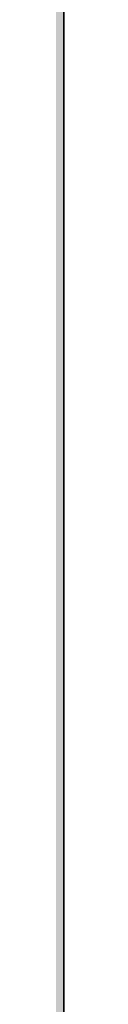
# Model space of a CAD drawing. Units: inches. Extents: x 2083 to 3317, y 1141 to 2115.
# Tile 185 of 256: x 3126.95978 to 3126.95979, y 1263.29018 to 1263.35483. Entities that reach past the tile are written whole.
import ezdxf

# ---------------------------------------------------------------- set-up
doc = ezdxf.new("R2010")
doc.units = ezdxf.units.IN
doc.layers.add('A-ANNO-DIMS', color=2, linetype='Continuous', lineweight=18)
doc.layers.add('A-WALL', color=7, linetype='Continuous', lineweight=35)
doc.layers.add('A-WALL-PATT', color=251, linetype='Continuous', lineweight=13, true_color=0x636466)
doc.styles.get("Standard").update_dxf_attribs({"font": 'arial.ttf'})
doc.dimstyles.new('ISO-25', dxfattribs={"dimtxt": 12, "dimasz": 12, "dimexe": 1.25, "dimexo": 0.625, "dimtad": 1, "dimlunit": 3, "dimtxsty": 'Standard', "dimcen": 2.5, "dimadec": 0, "dimazin": 0, "dimtfac": 1, "dimtmove": 0, "dimatfit": 3, "dimfxl": 1, "dimarcsym": 0})

# ---------------------------------------------------------------- blocks, each defined once
blk = doc.blocks.new('*D9')
at = {"layer": 'A-ANNO-DIMS', "color": 0, "lineweight": -2, "transparency": 16777216}
for p, q in [((3127.584783, 1486.76136), (3190.40309, 1486.76136)), ((3189.15309, 1474.76136), (3189.15309, 1275.26136)), ((3127.584783, 1263.26136), (3190.40309, 1263.26136))]:
    blk.add_line(p, q, dxfattribs=at)
at = {"layer": 'A-ANNO-DIMS', "color": 0, "transparency": 16777216}
for points in [[(3187.15309, 1474.76136), (3191.15309, 1474.76136), (3189.15309, 1486.76136)], [(3187.15309, 1275.26136), (3191.15309, 1275.26136), (3189.15309, 1263.26136)]]:
    blk.add_solid(points, dxfattribs=at)
at = {"layer": 'Defpoints', "color": 0, "transparency": 16777216}
for p in [(3126.959783, 1486.76136), (3126.959783, 1263.26136), (3189.15309, 1263.26136)]:
    blk.add_point(p, dxfattribs=at)
at = {"layer": 'A-ANNO-DIMS', "color": 0, "transparency": 16777216, "insert": (3182.401214, 1375.01136), "char_height": 12, "attachment_point": 5, "rotation": 90}
blk.add_mtext('18\'-7.5"', dxfattribs=at)
blk = doc.blocks.new('*D26')
at = {"layer": 'A-ANNO-DIMS', "color": 0, "lineweight": -2, "transparency": 16777216}
for p, q in [((3088.985844, 1274.915092), (3088.985844, 1270.951963)), ((3111.240037, 1274.915092), (3111.240037, 1270.951963)), ((3076.985844, 1272.201963), (2840.262447, 1272.201963)), ((3111.240037, 1272.201963), (3088.985844, 1272.201963)), ((3123.240037, 1272.201963), (3135.240037, 1272.201963))]:
    blk.add_line(p, q, dxfattribs=at)
at = {"layer": 'A-ANNO-DIMS', "color": 0, "transparency": 16777216}
for points in [[(3076.985844, 1274.201963), (3076.985844, 1270.201963), (3088.985844, 1272.201963)], [(3123.240037, 1274.201963), (3123.240037, 1270.201963), (3111.240037, 1272.201963)]]:
    blk.add_solid(points, dxfattribs=at)
at = {"layer": 'Defpoints', "color": 0, "transparency": 16777216}
for p in [(3088.985844, 1275.540092), (3111.240037, 1275.540092), (3088.985844, 1272.201963)]:
    blk.add_point(p, dxfattribs=at)
at = {"layer": 'A-ANNO-DIMS', "color": 0, "transparency": 16777216, "insert": (2952.624146, 1279.031602), "char_height": 12, "attachment_point": 5}
blk.add_mtext('NIGHTSTAND 1\'-10 1/2" TYP.', dxfattribs=at)
blk = doc.blocks.new('*D27')
at = {"layer": 'A-ANNO-DIMS', "color": 0, "lineweight": -2, "transparency": 16777216}
for p, q in [((3114.578165, 1309.794285), (3114.578165, 1321.794285)), ((3111.865037, 1297.794285), (3115.828165, 1297.794285)), ((3114.578165, 1297.794285), (3114.578165, 1275.540092)), ((3111.865037, 1275.540092), (3115.828165, 1275.540092)), ((3114.578165, 1263.540092), (3114.578165, 1140.988591))]:
    blk.add_line(p, q, dxfattribs=at)
at = {"layer": 'A-ANNO-DIMS', "color": 0, "transparency": 16777216}
for points in [[(3112.578165, 1309.794285), (3116.578165, 1309.794285), (3114.578165, 1297.794285)], [(3112.578165, 1263.540092), (3116.578165, 1263.540092), (3114.578165, 1275.540092)]]:
    blk.add_solid(points, dxfattribs=at)
at = {"layer": 'Defpoints', "color": 0, "transparency": 16777216}
for p in [(3111.240037, 1297.794285), (3111.240037, 1275.540092), (3114.578165, 1275.540092)]:
    blk.add_point(p, dxfattribs=at)
at = {"layer": 'A-ANNO-DIMS', "color": 0, "transparency": 16777216, "insert": (3107.748527, 1196.264342), "char_height": 12, "attachment_point": 5, "rotation": 90}
blk.add_mtext('1\'-10 1/2" TYP.', dxfattribs=at)

msp = doc.modelspace()

# ---------------------------------------------------------------- hatches: boundary and pattern name
at = {"layer": 'A-WALL-PATT'}
h = msp.add_hatch(color=256, dxfattribs=at)
h.dxf.hatch_style = 1
h.paths.add_polyline_path([(3126.959783, 2020.76136), (2748.959783, 2020.76136), (2604.959783, 2020.76136), (2226.959783, 2020.76136), (2226.959783, 1702.76136), (2466.959783, 1702.76136), (2466.959783, 1582.76136), (2418.959783, 1582.76136), (2418.959783, 1477.76136), (2226.959783, 1477.76136), (2226.959783, 1263.26136), (2544.959783, 1263.26136), (2544.959783, 1411.76136), (2604.959783, 1411.76136), (2685.959783, 1411.76136), (2685.959783, 1420.76136), (2604.959783, 1420.76136), (2604.959783, 1573.76136), (2604.959783, 1702.76136), (2604.959783, 2011.76136), (2748.959783, 2011.76136), (2748.959783, 1702.76136), (2862.959783, 1702.76136), (2862.959783, 1621.76136), (2871.959783, 1621.76136), (2871.959783, 1702.76136), (2883.959783, 1702.76136), (2883.959783, 1706.939459, -0.026459), (2883.959783, 1711.76136), (2757.959783, 1711.76136), (2757.959783, 1807.76136), (2787.959783, 1807.76136), (2787.959783, 1812.26136), (2757.959783, 1812.26136), (2757.959783, 2011.76136), (2877.959783, 2011.76136), (2877.959783, 1812.26136), (2847.959783, 1812.26136), (2847.959783, 1807.76136), (2889.835742, 1807.76136), (2889.835742, 1812.26136), (2882.459783, 1812.26136), (2882.459783, 2011.76136), (3117.959783, 2011.76136), (3117.959783, 1812.26136), (2937.835742, 1812.26136), (2937.835742, 1807.76136), (2995.709783, 1807.76136), (2995.709783, 1796.117666), (3000.209783, 1796.117666), (3000.209783, 1807.76136), (3117.959783, 1807.76136), (3117.959783, 1711.76136), (3000.209783, 1711.76136), (3000.209783, 1760.117666), (2998.572705, 1760.117666, -0.020711), (2995.709783, 1760.117666), (2995.709783, 1711.76136), (2931.959783, 1711.76136), (2931.959783, 1702.76136), (3126.959783, 1702.76136)])
h.paths.add_polyline_path([(2471.459783, 2011.76136), (2471.459783, 1810.01136), (2462.716936, 1810.01136), (2462.716936, 1805.51136), (2505.959783, 1805.51136), (2505.959783, 1810.01136), (2475.959783, 1810.01136), (2475.959783, 2011.76136), (2595.959783, 2011.76136), (2595.959783, 1810.01136), (2565.959783, 1810.01136), (2565.959783, 1805.51136), (2595.959783, 1805.51136), (2595.959783, 1711.76136), (2235.959783, 1711.76136), (2235.959783, 1805.51136), (2353.709783, 1805.51136), (2353.709783, 1796.054162), (2358.209783, 1796.054162), (2358.209783, 1805.51136), (2414.716936, 1805.51136), (2414.716936, 1810.01136), (2235.959783, 1810.01136), (2235.959783, 2011.76136)], flags=16)
h.paths.add_polyline_path([(2270.204734, 1994.610008), (2270.204734, 1970.610008), (2246.204734, 1970.610008), (2246.204734, 1994.610008)], flags=0)
edge = h.paths.add_edge_path(flags=0)
edge.add_ellipse((2332.027391, 1899.798176), major_axis=(-3.042994, 3.042994), ratio=0.16825245, start_angle=-161.332166, end_angle=-156.307114, ccw=False)
edge.add_ellipse((2333.082037, 1898.74353), major_axis=(-1.054646, 1.054646), ratio=0.4535321, start_angle=-123.371019, end_angle=-94.159107)
edge = h.paths.add_edge_path(flags=0)
edge.add_ellipse((2332.027391, 1968.87629), major_axis=(3.042994, 3.042994), ratio=0.16825245, start_angle=18.667834, end_angle=23.692886)
edge.add_spline(control_points=[(2332.925596, 1970.691105), (2332.226768, 1970.3361), (2330.893709, 1969.658905), (2328.41308, 1970.932138), (2327.203934, 1967.748712), (2324.709596, 1969.955589), (2322.532822, 1967.012354), (2320.012846, 1971.295812), (2317.680308, 1968.157845), (2316.040526, 1967.102047), (2315.426904, 1966.809602)], knot_values=[0, 0, 0, 0, 2.267059, 4.324559, 6.685584, 8.878641, 11.121502, 14.300359, 17.755284, 19.732645, 19.732645, 19.732645, 19.732645], degree=3, periodic=0)
edge.add_ellipse((2332.027391, 1968.87629), major_axis=(3.042994, 3.042994), ratio=0.16825245, start_angle=18.667834, end_angle=23.692886, ccw=False)
edge.add_ellipse((2333.082037, 1969.930936), major_axis=(1.054646, 1.054646), ratio=0.4535321, start_angle=56.628981, end_angle=85.840893, ccw=False)
edge = h.paths.add_edge_path(flags=0)
edge.add_spline(control_points=[(2296.428287, 1967.987908), (2293.627804, 1965.336314), (2287.703624, 1959.727094), (2299.74386, 1949.995699), (2294.532591, 1935.668528), (2290.573228, 1920.603512), (2293.394124, 1909.973691), (2296.185407, 1904.966543)], knot_values=[0.099185, 0.099185, 0.099185, 0.099185, 0.345301, 0.619822, 0.982653, 1.386093, 1.810555, 1.810555, 1.810555, 1.810555], degree=3, periodic=0)
edge.add_spline(control_points=[(2296.185407, 1904.966543), (2297.383582, 1902.6193), (2298.000969, 1901.949312), (2298.55297, 1901.468155)], knot_values=[0.006246, 0.006246, 0.006246, 0.006246, 0.055476, 0.055476, 0.055476, 0.055476], degree=3, periodic=0)
edge.add_spline(control_points=[(2298.55297, 1901.468155), (2297.258612, 1900.923224), (2295.225294, 1900.232126), (2293.060229, 1900.614205), (2292.101423, 1900.788415), (2292.089578, 1900.790568)], knot_values=[0.312835, 0.312835, 0.312835, 0.312835, 0.40178, 0.474987, 0.475903, 0.475903, 0.475903, 0.475903], degree=3, periodic=0)
edge.add_arc((2292.793646, 1904.664109), 3.937008, 215.420897, 259.698179, ccw=False)
edge.add_spline(control_points=[(2289.585314, 1902.382304), (2289.476652, 1902.535087), (2289.36848, 1902.688035), (2289.260865, 1902.84117)], knot_values=[0.102872, 0.102872, 0.102872, 0.102872, 0.116896, 0.116896, 0.116896, 0.116896], degree=3, periodic=0)
edge.add_spline(control_points=[(2289.260865, 1902.84117), (2288.686604, 1902.550192), (2287.640048, 1902.019902), (2285.881337, 1901.873954), (2283.852972, 1901.504352), (2281.719987, 1899.710538), (2278.466991, 1899.492942), (2276.157136, 1901.883202), (2272.258953, 1899.804071), (2267.777605, 1901.843183), (2262.243882, 1900.184033), (2257.414927, 1901.782061), (2254.318374, 1900.72612), (2253.178285, 1900.337343)], knot_values=[0, 0, 0, 0, 1.907977, 3.477176, 5.261074, 7.972851, 11.680248, 13.717921, 16.939592, 22.789562, 27.502503, 33.595215, 37.145618, 37.145618, 37.145618, 37.145618], degree=3, periodic=0)
edge.add_line((2253.178285, 1900.337343), (2250.24424, 1902.84117))
edge.add_line((2250.24424, 1902.84117), (2250.24424, 1965.833296))
edge.add_line((2250.24424, 1965.833296), (2253.178285, 1968.337123))
edge.add_spline(control_points=[(2253.178285, 1968.337123), (2254.318374, 1967.948346), (2257.414927, 1966.892405), (2262.243882, 1968.490433), (2267.777605, 1966.831283), (2271.52673, 1968.537217), (2273.875914, 1967.828289), (2274.206701, 1967.727642)], knot_values=[0, 0, 0, 0, 0.09018, 0.244935, 0.364644, 0.513233, 0.537855, 0.537855, 0.537855, 0.537855], degree=3, periodic=0)
edge.add_arc((2274.352887, 1963.793349), 3.937008, 72.051134, 92.127949, ccw=False)
edge.add_arc((2281.296933, 1985.230003), 18.596298, 252.0511336, 288.5657217)
edge.add_arc((2292.316717, 1956.02888), 12.646081, 71.0267879, 113.7782184, ccw=False)
edge = h.paths.add_edge_path(flags=0)
edge.add_spline(control_points=[(2274.899415, 1951.856195), (2275.066156, 1951.616592), (2275.232687, 1951.376588), (2275.397987, 1951.135855)], knot_values=[1.409916, 1.409916, 1.409916, 1.409916, 1.43159, 1.43159, 1.43159, 1.43159], degree=3, periodic=0)
edge.add_spline(control_points=[(2275.397987, 1951.135855), (2275.792106, 1950.561885), (2276.179231, 1949.983774), (2276.545546, 1949.397103)], knot_values=[1.358238, 1.358238, 1.358238, 1.358238, 1.409916, 1.409916, 1.409916, 1.409916], degree=3, periodic=0)
edge.add_line((2276.545546, 1949.397103), (2277.437289, 1947.862185))
edge.add_spline(control_points=[(2277.437289, 1947.862185), (2276.303834, 1945.673115), (2274.639698, 1942.426882), (2274.631615, 1938.0939), (2272.799124, 1930.85155), (2274.356426, 1943.897046), (2275.947681, 1947.923356), (2276.545546, 1949.397103)], knot_values=[0.005632, 0.005632, 0.005632, 0.005632, 0.186014, 0.266002, 0.357087, 0.59639, 0.739732, 0.739732, 0.739732, 0.739732], degree=3, periodic=0)
edge.add_spline(control_points=[(2276.545546, 1949.397103), (2276.179231, 1949.983774), (2275.792106, 1950.561885), (2275.397987, 1951.135855)], knot_values=[1.358238, 1.358238, 1.358238, 1.358238, 1.409916, 1.409916, 1.409916, 1.409916], degree=3, periodic=0)
edge.add_spline(control_points=[(2275.397987, 1951.135855), (2274.9425, 1950.080452), (2274.20776, 1948.025272), (2273.934602, 1944.851477), (2272.468534, 1937.627489), (2273.466216, 1945.696466), (2274.700615, 1951.059472), (2274.899415, 1951.856195)], knot_values=[0.104364, 0.104364, 0.104364, 0.104364, 0.189636, 0.269624, 0.36071, 0.600013, 0.644622, 0.644622, 0.644622, 0.644622], degree=3, periodic=0)
h.paths.add_polyline_path([(2269.167514, 1963.127573, -0.357527), (2268.170633, 1960.97637, -0.092561), (2268.170633, 1939.436325, -0.357527), (2269.167514, 1937.285122, -0.357527), (2267.01631, 1938.282002, -0.164785), (2254.685581, 1938.282002, -0.357527), (2252.534378, 1937.285122, -0.357527), (2253.531259, 1939.436325, -0.092561), (2253.531259, 1960.97637, -0.357527), (2252.534378, 1963.127573, -0.357527), (2254.685581, 1962.130692, -0.164785), (2267.01631, 1962.130692, -0.357527)], flags=0)
h.paths.add_polyline_path([(2248.874068, 1967.8018), (2248.874068, 1957.02771), (2249.457783, 1957.02771), (2249.457783, 1911.646756), (2248.874068, 1911.646756), (2248.874068, 1900.872666), (2246.511863, 1900.872666, 0.197327), (2244.149658, 1902.456873), (2244.149658, 1966.217592, 0.197327), (2246.511863, 1967.8018)], flags=0)
h.paths.add_polyline_path([(2269.167514, 1931.389344, -0.357527), (2268.170633, 1929.238141, -0.092561), (2268.170633, 1907.698096, -0.357527), (2269.167514, 1905.546893, -0.357527), (2267.01631, 1906.543774, -0.164785), (2254.685581, 1906.543774, -0.357527), (2252.534378, 1905.546893, -0.357527), (2253.531259, 1907.698096, -0.092561), (2253.531259, 1929.238141, -0.357527), (2252.534378, 1931.389344, -0.357527), (2254.685581, 1930.392463, -0.164785), (2267.01631, 1930.392463, -0.357527)], flags=0)
edge = h.paths.add_edge_path(flags=0)
edge.add_spline(control_points=[(2276.196858, 1906.723702), (2276.168144, 1909.028928), (2276.114049, 1913.371852), (2270.598417, 1924.924978), (2273.905175, 1919.012779), (2275.921711, 1916.262063), (2275.47457, 1912.402149), (2277.257874, 1910.380621), (2276.696044, 1908.225036), (2276.646218, 1906.813023), (2276.617825, 1906.008407)], knot_values=[0, 0, 0, 0, 8.61026, 16.221274, 18.843057, 23.804898, 27.440828, 29.356102, 31.203478, 33.650687, 33.650687, 33.650687, 33.650687], degree=3, periodic=0)
edge.add_spline(control_points=[(2276.617825, 1906.008407), (2276.623313, 1905.624144), (2276.497738, 1904.628661), (2275.441779, 1903.854725), (2274.937314, 1903.08045), (2274.85908, 1902.84117)], knot_values=[0.156488, 0.156488, 0.156488, 0.156488, 0.184398, 0.231376, 0.250598, 0.250598, 0.250598, 0.250598], degree=3, periodic=0)
edge.add_line((2274.85908, 1902.84117), (2276.50598, 1902.84117))
edge.add_spline(control_points=[(2276.50598, 1902.84117), (2276.788308, 1903.08494), (2277.665071, 1904.125196), (2278.249538, 1904.340738), (2277.653872, 1908.527387), (2278.15567, 1906.227808), (2278.100464, 1905.285948), (2278.846675, 1904.069005), (2277.856785, 1903.414948), (2277.874191, 1902.99105), (2277.903562, 1902.84117)], knot_values=[0.059574, 0.059574, 0.059574, 0.059574, 0.080753, 0.103741, 0.16972, 0.176036, 0.207137, 0.240474, 0.262341, 0.27366, 0.27366, 0.27366, 0.27366], degree=3, periodic=0)
edge.add_line((2277.903562, 1902.84117), (2280.029825, 1902.84117))
edge.add_spline(control_points=[(2280.029825, 1902.84117), (2279.888221, 1903.088398), (2279.499257, 1903.981551), (2280.152284, 1905.939349), (2278.103615, 1909.657757), (2279.762395, 1907.185285), (2280.3279, 1904.874861), (2280.485109, 1903.48959), (2281.463269, 1903.249432), (2281.758343, 1902.936497), (2281.834036, 1902.84117)], knot_values=[0.013856, 0.013856, 0.013856, 0.013856, 0.034874, 0.088867, 0.107879, 0.126738, 0.158714, 0.193757, 0.217487, 0.226722, 0.226722, 0.226722, 0.226722], degree=3, periodic=0)
edge.add_spline(control_points=[(2281.834036, 1902.84117), (2281.787535, 1902.826703), (2281.647022, 1902.782988), (2281.395527, 1902.85949), (2281.088077, 1902.985242), (2280.720683, 1903.060902), (2280.333451, 1903.025726), (2280.124767, 1902.898879), (2280.029825, 1902.84117)], knot_values=[0, 0, 0, 0, 0.14413, 0.435517, 0.749276, 1.153046, 1.548371, 1.878348, 1.878348, 1.878348, 1.878348], degree=3, periodic=0)
edge.add_line((2280.029825, 1902.84117), (2277.903562, 1902.84117))
edge.add_spline(control_points=[(2277.903562, 1902.84117), (2277.892855, 1902.795855), (2277.865396, 1902.679637), (2277.607479, 1902.687483), (2277.27405, 1902.8007), (2276.837921, 1902.619775), (2276.583807, 1902.789261), (2276.50598, 1902.84117)], knot_values=[0, 0, 0, 0, 0.127189, 0.326199, 0.628009, 1.24357, 1.515331, 1.515331, 1.515331, 1.515331], degree=3, periodic=0)
edge.add_line((2276.50598, 1902.84117), (2274.85908, 1902.84117))
edge.add_spline(control_points=[(2274.85908, 1902.84117), (2274.814437, 1902.898587), (2274.72513, 1903.013446), (2274.493477, 1903.118968), (2274.244285, 1902.960539), (2273.937121, 1903.184942), (2273.614039, 1902.983143), (2273.408316, 1902.883045), (2273.322254, 1902.84117)], knot_values=[0, 0, 0, 0, 0.21843, 0.436957, 0.687977, 0.990379, 1.398396, 1.69185, 1.69185, 1.69185, 1.69185], degree=3, periodic=0)
edge.add_spline(control_points=[(2273.322254, 1902.84117), (2273.61674, 1903.445692), (2274.273998, 1904.538253), (2276.027239, 1904.573702), (2276.206963, 1906.583637), (2276.196858, 1906.723702)], knot_values=[0.012227, 0.012227, 0.012227, 0.012227, 0.059472, 0.106218, 0.134458, 0.134458, 0.134458, 0.134458], degree=3, periodic=0)
h.paths.add_polyline_path([(2270.776054, 1897.789828), (2270.776054, 1873.789828), (2246.776054, 1873.789828), (2246.776054, 1897.789828)], flags=0)
h.paths.add_polyline_path([(2353.709783, 1760.005059), (2353.709783, 1760.054162), (2358.209783, 1760.054162, -0.033729)], flags=0)
h.paths.add_polyline_path([(2321.819119, 1737.529186), (2341.995327, 1737.529186, -0.414214), (2343.203273, 1736.321241), (2343.203273, 1721.020596, -0.414214), (2341.995327, 1719.812651), (2321.819119, 1719.812651, -0.414214), (2320.611173, 1721.020596), (2320.611173, 1736.321241, -0.414214)], flags=0)
h.paths.add_polyline_path([(2324.23501, 1736.321241), (2339.579436, 1736.321241, -0.414214), (2341.995327, 1733.905349), (2341.995327, 1725.44973, -0.414214), (2339.579436, 1723.033839), (2333.680588, 1723.033839), (2333.845317, 1722.045467, -0.870646), (2335.425399, 1721.825893, -0.767327), (2333.922694, 1721.423245), (2331.291024, 1721.423245, -0.767327), (2329.788319, 1721.825893, -0.870646), (2331.368401, 1722.045467), (2331.53313, 1723.033839), (2324.23501, 1723.033839, -0.414214), (2321.819119, 1725.44973), (2321.819119, 1733.905349, -0.414214)], flags=0)
h.paths.add_polyline_path([(2570.483789, 1928.615444), (2589.683789, 1928.615444), (2590.168829, 1928.615444), (2590.168829, 1904.993397), (2570.483789, 1904.993397)], flags=0)
h.paths.add_polyline_path([(2574.447324, 1927.263822, -1), (2572.828836, 1927.263822, -1)], flags=0)
h.paths.add_polyline_path([(2573.089867, 1926.940877), (2573.925032, 1927.776042), (2574.147743, 1927.553332), (2573.312577, 1926.718166)], flags=0)
h.paths.add_polyline_path([(2578.779065, 1919.729618, -1), (2571.591663, 1919.729618, -1)], flags=0)
h.paths.add_polyline_path([(2578.385364, 1919.729618, -1), (2571.985364, 1919.729618, -1)], flags=0)
h.paths.add_polyline_path([(2331.595764, 1729.476216, -1), (2333.617954, 1729.476216, -1)], flags=0)
h.paths.add_polyline_path([(2578.034228, 1927.263822, -1), (2576.41574, 1927.263822, -1)], flags=0)
h.paths.add_polyline_path([(2576.688851, 1927.531089), (2576.911562, 1927.753799), (2577.746728, 1926.918634), (2577.524017, 1926.695923)], flags=0)
h.paths.add_polyline_path([(2578.139065, 1909.859539, -1), (2572.231663, 1909.859539, -1)], flags=0)
h.paths.add_polyline_path([(2577.745364, 1909.859539, -1), (2572.625364, 1909.859539, -1)], flags=0)
h.paths.add_polyline_path([(2583.797718, 1927.263822, -1), (2582.179229, 1927.263822, -1)], flags=0)
h.paths.add_polyline_path([(2582.718649, 1927.753799), (2583.553814, 1926.918634), (2583.331103, 1926.695923), (2582.495938, 1927.531089)], flags=0)
h.paths.add_polyline_path([(2582.495938, 1927.531089), (2582.718649, 1927.753799), (2583.553814, 1926.918634), (2583.331103, 1926.695923)], flags=0)
h.paths.add_polyline_path([(2587.739065, 1920.529618, -1), (2581.831663, 1920.529618, -1)], flags=0)
h.paths.add_polyline_path([(2587.345364, 1920.529618, -1), (2582.225364, 1920.529618, -1)], flags=0)
h.paths.add_polyline_path([(2587.384622, 1927.263822, -1), (2585.766133, 1927.263822, -1)], flags=0)
h.paths.add_polyline_path([(2586.081993, 1926.980247), (2586.917158, 1927.815412), (2587.139869, 1927.592702), (2586.304703, 1926.757536)], flags=0)
h.paths.add_polyline_path([(2588.379065, 1910.659539, -1), (2581.191663, 1910.659539, -1)], flags=0)
h.paths.add_polyline_path([(2587.985364, 1910.659539, -1), (2581.585364, 1910.659539, -1)], flags=0)
h.paths.add_polyline_path([(2417.167729, 1729.477895), (2437.343937, 1729.477895, -0.414214), (2438.551883, 1728.26995), (2438.551883, 1712.969306, -0.414214), (2437.343937, 1711.76136), (2417.167729, 1711.76136, -0.414214), (2415.959783, 1712.969306), (2415.959783, 1728.26995, -0.414214)], flags=0)
h.paths.add_polyline_path([(2419.58362, 1728.26995), (2434.928046, 1728.26995, -0.414214), (2437.343937, 1725.854059), (2437.343937, 1717.39844, -0.414214), (2434.928046, 1714.982548), (2429.029199, 1714.982548), (2429.193927, 1713.994176, -0.870646), (2430.774009, 1713.774603, -0.767327), (2429.271304, 1713.371954), (2426.639634, 1713.371954, -0.767327), (2425.136929, 1713.774603, -0.870646), (2426.717011, 1713.994176), (2426.88174, 1714.982548), (2419.58362, 1714.982548, -0.414214), (2417.167729, 1717.39844), (2417.167729, 1725.854059, -0.414214)], flags=0)
h.paths.add_polyline_path([(2419.58362, 1728.26995), (2434.928046, 1728.26995, -0.414214), (2437.343937, 1725.854059), (2437.343937, 1717.39844, -0.414214), (2434.928046, 1714.982548), (2429.029199, 1714.982548), (2428.358118, 1719.009034), (2427.552821, 1719.009034), (2426.88174, 1714.982548), (2419.58362, 1714.982548, -0.414214), (2417.167729, 1717.39844), (2417.167729, 1725.854059, -0.414214)], flags=0)
h.paths.add_polyline_path([(2426.944374, 1721.424925, -1), (2428.966564, 1721.424925, -1)], flags=0)
h.paths.add_polyline_path([(2475.959783, 1702.76136), (2595.959783, 1702.76136), (2595.959783, 1582.76136), (2475.959783, 1582.76136)], flags=16)
h.paths.add_polyline_path([(2427.959783, 1573.76136), (2595.959783, 1573.76136), (2595.959783, 1468.76136), (2595.959783, 1420.76136), (2384.459783, 1420.76136), (2384.459783, 1468.76136), (2427.959783, 1468.76136)], flags=16)
h.paths.add_polyline_path([(2379.959783, 1468.76136), (2379.959783, 1420.76136), (2235.959783, 1420.76136), (2235.959783, 1468.76136)], flags=16)
h.paths.add_polyline_path([(2317.815996, 1466.695767), (2337.992205, 1466.695767, -0.414214), (2339.20015, 1465.487821), (2339.20015, 1450.187177, -0.414214), (2337.992205, 1448.979232), (2317.815996, 1448.979232, -0.414214), (2316.608051, 1450.187177), (2316.608051, 1465.487821, -0.414214)], flags=0)
h.paths.add_polyline_path([(2320.231887, 1465.487821), (2335.576313, 1465.487821, -0.414214), (2337.992205, 1463.07193), (2337.992205, 1454.616311, -0.414214), (2335.576313, 1452.20042), (2329.677466, 1452.20042), (2329.842195, 1451.212047, -0.870646), (2331.422276, 1450.992474, -0.767327), (2329.919571, 1450.589826), (2327.287902, 1450.589826, -0.767327), (2325.785197, 1450.992474, -0.870646), (2327.365278, 1451.212047), (2327.530007, 1452.20042), (2320.231887, 1452.20042, -0.414214), (2317.815996, 1454.616311), (2317.815996, 1463.07193, -0.414214)], flags=0)
h.paths.add_polyline_path([(2320.231887, 1465.487821), (2335.576313, 1465.487821, -0.414214), (2337.992205, 1463.07193), (2337.992205, 1454.616311, -0.414214), (2335.576313, 1452.20042), (2329.677466, 1452.20042), (2329.006385, 1456.226905), (2328.201088, 1456.226905), (2327.530007, 1452.20042), (2320.231887, 1452.20042, -0.414214), (2317.815996, 1454.616311), (2317.815996, 1463.07193, -0.414214)], flags=0)
h.paths.add_polyline_path([(2327.592641, 1458.642796, -1), (2329.614832, 1458.642796, -1)], flags=0)
h.paths.add_polyline_path([(2244.411744, 1433.340453), (2241.920945, 1433.340453, -0.414214), (2240.017856, 1435.243542), (2240.017856, 1440.952808, -0.414211), (2241.920925, 1442.855897), (2244.411744, 1442.855897, -1.976472)], flags=0)
h.paths.add_polyline_path([(2245.356888, 1434.397536, -0.414214), (2245.356888, 1441.798814, -2.144098)], flags=0)
h.paths.add_polyline_path([(2535.959783, 1416.26136), (2535.959783, 1272.26136), (2235.959783, 1272.26136), (2235.959783, 1416.26136)], flags=16)
h.paths.add_polyline_path([(2260.119561, 1384.292841), (2260.119561, 1362.038649), (2237.865369, 1362.038649), (2237.865369, 1384.292841)], flags=0)
edge = h.paths.add_edge_path(flags=0)
edge.add_line((2318.251847, 1362.093298), (2318.145797, 1362.000973))
edge.add_ellipse((2317.445116, 1360.431044), major_axis=(2.82164, 2.82164), ratio=0.16825245, start_angle=18.667834, end_angle=20.948127, ccw=False)
edge.add_ellipse((2318.423045, 1361.408974), major_axis=(0.977929, 0.977929), ratio=0.4535321, start_angle=56.628981, end_angle=70.226201, ccw=False)
edge = h.paths.add_edge_path(flags=0)
edge.add_line((2319.10737, 1295.571078), (2319.015044, 1295.677128))
edge.add_ellipse((2317.445116, 1296.377809), major_axis=(-2.82164, 2.82164), ratio=0.16825245, start_angle=-161.332166, end_angle=-159.051873, ccw=False)
edge.add_ellipse((2318.423045, 1295.39988), major_axis=(-0.977929, 0.977929), ratio=0.4535321, start_angle=-123.371019, end_angle=-109.773799)
edge = h.paths.add_edge_path(flags=0)
edge.add_spline(control_points=[(2284.210349, 1301.170219), (2284.580688, 1300.444719), (2284.891189, 1299.892024), (2285.159553, 1299.461018)], knot_values=[0.039066, 0.039066, 0.039066, 0.039066, 0.055476, 0.055476, 0.055476, 0.055476], degree=3, periodic=0)
edge.add_line((2285.159553, 1299.461018), (2284.210349, 1301.170219))
edge = h.paths.add_edge_path(flags=0)
edge.add_line((2280.412458, 1297.298013), (2283.369991, 1297.036122))
edge.add_line((2283.369991, 1297.036122), (2286.40569, 1297.92631))
edge.add_spline(control_points=[(2286.40569, 1297.92631), (2285.305487, 1297.463119), (2284.344777, 1297.129151), (2283.369991, 1297.036122)], knot_values=[0.394369, 0.394369, 0.394369, 0.394369, 0.475903, 0.475903, 0.475903, 0.475903], degree=3, periodic=0)
edge.add_spline(control_points=[(2283.369991, 1297.036122), (2283.28139, 1297.027666), (2282.316289, 1296.957336), (2281.312502, 1297.134479), (2280.423441, 1297.296016), (2280.412458, 1297.298013)], knot_values=[0.312835, 0.312835, 0.312835, 0.312835, 0.320246, 0.393453, 0.394369, 0.394369, 0.394369, 0.394369], degree=3, periodic=0)
edge = h.paths.add_edge_path(flags=0)
edge.add_line((2284.435561, 1359.607285), (2280.446291, 1355.328047))
edge.add_line((2280.446291, 1355.328047), (2279.579987, 1351.017754))
edge.add_line((2279.579987, 1351.017754), (2282.412974, 1346.580433))
edge.add_spline(control_points=[(2282.412974, 1346.580433), (2283.153331, 1345.589236), (2284.252896, 1344.028897), (2284.801037, 1342.387167), (2284.935162, 1341.805544)], knot_values=[1.240098, 1.240098, 1.240098, 1.240098, 1.332892, 1.382712, 1.382712, 1.382712, 1.382712], degree=3, periodic=0)
edge.add_spline(control_points=[(2284.935162, 1341.805544), (2285.319108, 1340.1406), (2285.233029, 1338.409204), (2284.909938, 1336.654122)], knot_values=[1.097484, 1.097484, 1.097484, 1.097484, 1.240098, 1.240098, 1.240098, 1.240098], degree=3, periodic=0)
edge.add_spline(control_points=[(2284.909938, 1336.654122), (2284.586848, 1334.89904), (2284.026745, 1333.120272), (2283.462644, 1331.360585)], knot_values=[0.95487, 0.95487, 0.95487, 0.95487, 1.097484, 1.097484, 1.097484, 1.097484], degree=3, periodic=0)
edge.add_line((2283.462644, 1331.360585), (2281.890376, 1326.153357))
edge.add_line((2281.890376, 1326.153357), (2280.756259, 1321.056089))
edge.add_line((2280.756259, 1321.056089), (2280.299205, 1316.001977))
edge.add_line((2280.299205, 1316.001977), (2280.715933, 1310.950068))
edge.add_line((2280.715933, 1310.950068), (2282.028094, 1305.972137))
edge.add_line((2282.028094, 1305.972137), (2284.210349, 1301.170219))
edge.add_spline(control_points=[(2284.210349, 1301.170219), (2283.340731, 1302.730185), (2282.611904, 1304.336493), (2282.028094, 1305.972137)], knot_values=[0.099185, 0.099185, 0.099185, 0.099185, 0.241799, 0.241799, 0.241799, 0.241799], degree=3, periodic=0)
edge.add_spline(control_points=[(2282.028094, 1305.972137), (2281.444283, 1307.60778), (2281.005489, 1309.272759), (2280.715933, 1310.950068)], knot_values=[0.241799, 0.241799, 0.241799, 0.241799, 0.384413, 0.384413, 0.384413, 0.384413], degree=3, periodic=0)
edge.add_spline(control_points=[(2280.715933, 1310.950068), (2280.433241, 1312.587613), (2280.289386, 1314.276959), (2280.298894, 1315.962032), (2280.299205, 1316.001977)], knot_values=[0.384413, 0.384413, 0.384413, 0.384413, 0.523647, 0.527028, 0.527028, 0.527028, 0.527028], degree=3, periodic=0)
edge.add_spline(control_points=[(2280.299205, 1316.001977), (2280.312326, 1317.686955), (2280.477871, 1319.367926), (2280.756259, 1321.056089)], knot_values=[0.527028, 0.527028, 0.527028, 0.527028, 0.669642, 0.669642, 0.669642, 0.669642], degree=3, periodic=0)
edge.add_spline(control_points=[(2280.756259, 1321.056089), (2281.034648, 1322.744252), (2281.42588, 1324.439608), (2281.890376, 1326.153357)], knot_values=[0.669642, 0.669642, 0.669642, 0.669642, 0.812256, 0.812256, 0.812256, 0.812256], degree=3, periodic=0)
edge.add_spline(control_points=[(2281.890376, 1326.153357), (2282.264383, 1327.533251), (2282.78787, 1329.26181), (2283.352751, 1331.01778), (2283.462644, 1331.360585)], knot_values=[0.812256, 0.812256, 0.812256, 0.812256, 0.927087, 0.95487, 0.95487, 0.95487, 0.95487], degree=3, periodic=0)
edge.add_line((2283.462644, 1331.360585), (2284.909938, 1336.654122))
edge.add_line((2284.909938, 1336.654122), (2284.935162, 1341.805544))
edge.add_line((2284.935162, 1341.805544), (2282.412974, 1346.580433))
edge.add_spline(control_points=[(2282.412974, 1346.580433), (2281.275127, 1348.103792), (2280.078447, 1349.570318), (2279.579987, 1351.017754)], knot_values=[1.382712, 1.382712, 1.382712, 1.382712, 1.525326, 1.525326, 1.525326, 1.525326], degree=3, periodic=0)
edge.add_spline(control_points=[(2279.579987, 1351.017754), (2279.443282, 1351.414721), (2279.136312, 1352.856922), (2279.73519, 1354.290385), (2280.446291, 1355.328047)], knot_values=[1.525326, 1.525326, 1.525326, 1.525326, 1.564439, 1.667941, 1.667941, 1.667941, 1.667941], degree=3, periodic=0)
edge.add_spline(control_points=[(2280.446291, 1355.328047), (2281.426113, 1356.757835), (2282.930837, 1358.18256), (2284.435561, 1359.607285)], knot_values=[1.667941, 1.667941, 1.667941, 1.667941, 1.810555, 1.810555, 1.810555, 1.810555], degree=3, periodic=0)
edge.add_arc((2280.623075, 1348.518181), 11.72618, 71.0267879, 113.7782184)
edge.add_arc((2270.404892, 1375.595156), 17.243567, 252.0511336, 288.5657217, ccw=False)
edge.add_arc((2263.965969, 1355.717847), 3.650622, 72.051134, 92.127949)
edge.add_arc((2263.965969, 1355.717847), 3.650622, 92.127949, 177.98513)
edge.add_spline(control_points=[(2260.317604, 1355.846199), (2260.260417, 1354.220668), (2260.551278, 1350.186547), (2262.999344, 1346.766251), (2264.472741, 1344.649024)], knot_values=[1.43159, 1.43159, 1.43159, 1.43159, 1.564144, 1.770695, 1.770695, 1.770695, 1.770695], degree=3, periodic=0)
edge.add_line((2264.472741, 1344.649024), (2264.93559, 1343.98253))
edge.add_spline(control_points=[(2263.801044, 1340.248105), (2263.843238, 1340.514088), (2264.067244, 1341.756465), (2264.512693, 1343.002453), (2264.935047, 1343.981083)], knot_values=[0.53657, 0.53657, 0.53657, 0.53657, 0.559349, 0.644622, 0.644622, 0.644622, 0.644622], degree=3, periodic=0)
edge.add_spline(control_points=[(2264.935047, 1343.981083), (2265.117771, 1343.714975), (2265.298875, 1343.447906), (2265.476756, 1343.179365)], knot_values=[1.384077, 1.384077, 1.384077, 1.384077, 1.409916, 1.409916, 1.409916, 1.409916], degree=3, periodic=0)
edge.add_spline(control_points=[(2265.476756, 1343.179365), (2265.654637, 1342.910823), (2265.829296, 1342.64081), (2265.99913, 1342.368812)], knot_values=[1.358238, 1.358238, 1.358238, 1.358238, 1.384077, 1.384077, 1.384077, 1.384077], degree=3, periodic=0)
edge.add_line((2265.99913, 1342.368812), (2266.826006, 1340.945547))
edge.add_spline(control_points=[(2266.826006, 1340.945547), (2268.894401, 1337.089691), (2271.398173, 1325.843001), (2270.516164, 1310.568557), (2275.919376, 1301.860609), (2277.789511, 1299.19945)], knot_values=[0.116896, 0.116896, 0.116896, 0.116896, 0.472987, 1.050969, 1.313793, 1.313793, 1.313793, 1.313793], degree=3, periodic=0)
edge.add_spline(control_points=[(2277.789511, 1299.19945), (2277.839405, 1299.128452), (2277.889428, 1299.057498), (2277.939572, 1298.986584)], knot_values=[0.109884, 0.109884, 0.109884, 0.109884, 0.116896, 0.116896, 0.116896, 0.116896], degree=3, periodic=0)
edge.add_line((2277.939572, 1298.986584), (2277.788849, 1299.199114))
edge.add_spline(control_points=[(2277.788849, 1299.199114), (2277.256582, 1298.929414), (2276.28635, 1298.437902), (2275.039352, 1298.334419), (2274.38333, 1298.238895), (2274.215254, 1298.209338)], knot_values=[33.12187, 33.12187, 33.12187, 33.12187, 35.029056, 36.598255, 37.144827, 37.144827, 37.144827, 37.144827], degree=3, periodic=0)
edge.add_line((2274.215254, 1298.209338), (2273.073147, 1297.892961))
edge.add_spline(control_points=[(2273.073147, 1297.892961), (2272.322936, 1297.579784), (2271.039151, 1296.510508), (2269.248395, 1296.226062), (2268.4231, 1296.374654)], knot_values=[26.532584, 26.532584, 26.532584, 26.532584, 29.198919, 31.839101, 31.839101, 31.839101, 31.839101], degree=3, periodic=0)
edge.add_line((2268.4231, 1296.374654), (2263.878501, 1297.457534))
edge.add_spline(control_points=[(2263.878501, 1297.457534), (2263.556077, 1297.359435), (2261.860306, 1296.838694), (2260.23878, 1297.282407), (2258.933454, 1297.516461)], knot_values=[15.919551, 15.919551, 15.919551, 15.919551, 16.939592, 21.226067, 21.226067, 21.226067, 21.226067], degree=3, periodic=0)
edge.add_line((2258.933454, 1297.516461), (2254.055233, 1297.32901))
edge.add_spline(control_points=[(2254.055233, 1297.32901), (2253.755525, 1297.295815), (2252.113683, 1297.165174), (2250.461869, 1297.544221), (2249.129686, 1297.667882)], knot_values=[5.306517, 5.306517, 5.306517, 5.306517, 6.276435, 10.613034, 10.613034, 10.613034, 10.613034], degree=3, periodic=0)
edge.add_line((2249.129686, 1297.667882), (2244.33165, 1296.877756))
edge.add_line((2244.33165, 1296.877756), (2241.611033, 1299.19945))
edge.add_line((2241.611033, 1299.19945), (2241.611033, 1357.609404))
edge.add_line((2241.611033, 1357.609404), (2244.33165, 1359.931097))
edge.add_line((2244.33165, 1359.931097), (2252.728823, 1359.542692))
edge.add_spline(control_points=[(2252.728823, 1359.542692), (2252.870939, 1359.54644), (2253.30574, 1359.548172), (2253.739845, 1359.514274), (2254.031742, 1359.482426)], knot_values=[0.233291, 0.233291, 0.233291, 0.233291, 0.244935, 0.268927, 0.268927, 0.268927, 0.268927], degree=3, periodic=0)
edge.add_line((2254.031742, 1359.482426), (2259.58719, 1359.41639))
edge.add_spline(control_points=[(2259.58719, 1359.41639), (2260.677068, 1359.628503), (2262.073197, 1359.897003), (2263.523692, 1359.459278), (2263.830417, 1359.365952)], knot_values=[0.422516, 0.422516, 0.422516, 0.422516, 0.513233, 0.537855, 0.537855, 0.537855, 0.537855], degree=3, periodic=0)
edge.add_arc((2263.965969, 1355.717847), 3.650622, 72.051134, 92.127949, ccw=False)
edge.add_arc((2270.404892, 1375.595156), 17.243567, 252.0511336, 288.5657217)
edge.add_arc((2280.623075, 1348.518181), 11.72618, 71.0267879, 113.7782184, ccw=False)
h.paths.add_polyline_path([(2240.34053, 1359.434715), (2240.34053, 1349.444353), (2240.881785, 1349.444353), (2240.881785, 1307.3645), (2240.34053, 1307.3645), (2240.34053, 1297.374138), (2238.150157, 1297.374138, 0.197327), (2235.959783, 1298.843108), (2235.959783, 1357.965746, 0.197327), (2238.150157, 1359.434715)], flags=0)
h.paths.add_polyline_path([(2259.15779, 1355.1005, -0.357527), (2258.233425, 1353.10578, -0.092561), (2258.233425, 1333.132601, -0.357527), (2259.15779, 1331.13788, -0.357527), (2257.16307, 1332.062246, -0.164785), (2245.729302, 1332.062246, -0.357527), (2243.734582, 1331.13788, -0.357527), (2244.658947, 1333.132601, -0.092561), (2244.658947, 1353.10578, -0.357527), (2243.734582, 1355.1005, -0.357527), (2245.729302, 1354.176135, -0.164785), (2257.16307, 1354.176135, -0.357527)], flags=0)
edge = h.paths.add_edge_path(flags=0)
edge.add_line((2265.99913, 1342.368812), (2266.826006, 1340.945547))
edge.add_line((2266.826006, 1340.945547), (2265.307557, 1337.814066))
edge.add_line((2265.307557, 1337.814066), (2264.358232, 1334.652939))
edge.add_line((2264.358232, 1334.652939), (2264.262012, 1333.799705))
edge.add_spline(control_points=[(2264.262012, 1333.799705), (2264.208357, 1333.187055), (2264.16206, 1332.365525), (2264.007144, 1331.413933), (2263.969049, 1331.201834)], knot_values=[0.464444, 0.464444, 0.464444, 0.464444, 0.516691, 0.531608, 0.531608, 0.531608, 0.531608], degree=3, periodic=0)
edge.add_spline(control_points=[(2263.969049, 1331.201834), (2263.774535, 1330.118873), (2263.42437, 1328.790839), (2263.25742, 1328.530652), (2263.234028, 1328.514612)], knot_values=[0.372682, 0.372682, 0.372682, 0.372682, 0.44885, 0.464444, 0.464444, 0.464444, 0.464444], degree=3, periodic=0)
edge.add_spline(control_points=[(2263.234028, 1328.514612), (2263.096382, 1328.420227), (2263.13117, 1329.301477), (2263.274953, 1330.615749)], knot_values=[0.280919, 0.280919, 0.280919, 0.280919, 0.372682, 0.372682, 0.372682, 0.372682], degree=3, periodic=0)
edge.add_spline(control_points=[(2263.274953, 1330.615749), (2263.418736, 1331.930022), (2263.671515, 1333.677318), (2263.969852, 1335.315027)], knot_values=[0.189157, 0.189157, 0.189157, 0.189157, 0.280919, 0.280919, 0.280919, 0.280919], degree=3, periodic=0)
edge.add_spline(control_points=[(2263.969852, 1335.315027), (2264.100496, 1336.032192), (2264.418783, 1337.621911), (2264.754848, 1338.86443), (2264.947419, 1339.491124)], knot_values=[0.097394, 0.097394, 0.097394, 0.097394, 0.137578, 0.189157, 0.189157, 0.189157, 0.189157], degree=3, periodic=0)
edge.add_spline(control_points=[(2264.947419, 1339.491124), (2265.290017, 1340.606055), (2265.644238, 1341.493996), (2265.99913, 1342.368812)], knot_values=[0.005632, 0.005632, 0.005632, 0.005632, 0.097394, 0.097394, 0.097394, 0.097394], degree=3, periodic=0)
h.paths.add_polyline_path([(2259.15779, 1325.670973, -0.357527), (2258.233425, 1323.676253, -0.092561), (2258.233425, 1303.703073, -0.357527), (2259.15779, 1301.708353, -0.357527), (2257.16307, 1302.632719, -0.164785), (2245.729302, 1302.632719, -0.357527), (2243.734582, 1301.708353, -0.357527), (2244.658947, 1303.703073, -0.092561), (2244.658947, 1323.676253, -0.357527), (2243.734582, 1325.670973, -0.357527), (2245.729302, 1324.746608, -0.164785), (2257.16307, 1324.746608, -0.357527)], flags=0)
edge = h.paths.add_edge_path(flags=0)
edge.add_spline(control_points=[(2261.708938, 1317.311421), (2261.679482, 1317.41758), (2261.761858, 1317.388535), (2262.490736, 1316.089873), (2262.962185, 1315.300897)], knot_values=[14.955861, 14.955861, 14.955861, 14.955861, 16.221274, 18.694826, 18.694826, 18.694826, 18.694826], degree=3, periodic=0)
edge.add_spline(control_points=[(2262.962185, 1315.300897), (2262.990437, 1315.253617), (2263.702096, 1314.067376), (2264.348983, 1313.127153), (2264.730054, 1312.164154)], knot_values=[18.694826, 18.694826, 18.694826, 18.694826, 18.843057, 22.433791, 22.433791, 22.433791, 22.433791], degree=3, periodic=0)
edge.add_spline(control_points=[(2264.730054, 1312.164154), (2264.875565, 1311.796437), (2265.176873, 1310.769807), (2265.143069, 1309.559262), (2265.247736, 1308.824193)], knot_values=[22.433791, 22.433791, 22.433791, 22.433791, 23.804898, 26.172756, 26.172756, 26.172756, 26.172756], degree=3, periodic=0)
edge.add_line((2265.247736, 1308.824193), (2265.850774, 1307.171888))
edge.add_spline(control_points=[(2265.850774, 1307.171888), (2266.065025, 1306.821678), (2266.384387, 1306.332246), (2266.4244, 1305.780549), (2266.420369, 1305.611216)], knot_values=[28.062562, 28.062562, 28.062562, 28.062562, 29.356102, 29.911721, 29.911721, 29.911721, 29.911721], degree=3, periodic=0)
edge.add_spline(control_points=[(2266.420369, 1305.611216), (2266.416116, 1305.43259), (2266.393999, 1305.249998), (2266.364777, 1305.065857)], knot_values=[29.911721, 29.911721, 29.911721, 29.911721, 30.497837, 30.497837, 30.497837, 30.497837], degree=3, periodic=0)
edge.add_line((2266.364777, 1305.065857), (2266.066151, 1302.136295))
edge.add_spline(control_points=[(2266.066151, 1302.136295), (2266.07124, 1301.779984), (2265.998076, 1301.199985), (2265.663266, 1300.758961), (2265.508908, 1300.585882)], knot_values=[0.156488, 0.156488, 0.156488, 0.156488, 0.184398, 0.203543, 0.203543, 0.203543, 0.203543], degree=3, periodic=0)
edge.add_line((2265.508908, 1300.585882), (2264.435341, 1299.19945))
edge.add_line((2264.435341, 1299.19945), (2265.962442, 1299.19945))
edge.add_line((2265.962442, 1299.19945), (2267.33599, 1301.175276))
edge.add_line((2267.33599, 1301.175276), (2267.311667, 1301.986237))
edge.add_spline(control_points=[(2267.311667, 1301.986237), (2267.261111, 1302.862396), (2267.160212, 1303.737132), (2267.271486, 1303.325896)], knot_values=[0.126229, 0.126229, 0.126229, 0.126229, 0.166617, 0.166617, 0.166617, 0.166617], degree=3, periodic=0)
edge.add_spline(control_points=[(2267.271486, 1303.325896), (2267.280035, 1303.294305), (2267.309785, 1303.175366), (2267.37345, 1302.883608), (2267.406123, 1302.682829), (2267.417926, 1302.601025)], knot_values=[0.166617, 0.166617, 0.166617, 0.166617, 0.16972, 0.176036, 0.180765, 0.180765, 0.180765, 0.180765], degree=3, periodic=0)
edge.add_spline(control_points=[(2267.743891, 1300.987505), (2267.687583, 1301.150943), (2267.48052, 1301.656664), (2267.483751, 1302.144788), (2267.417926, 1302.601025)], knot_values=[0.180765, 0.180765, 0.180765, 0.180765, 0.193767, 0.220139, 0.220139, 0.220139, 0.220139], degree=3, periodic=0)
edge.add_line((2267.417926, 1302.601025), (2267.743891, 1300.987505))
edge.add_spline(control_points=[(2267.743891, 1300.987505), (2267.831961, 1300.731878), (2267.932021, 1300.309904), (2267.554841, 1299.974518), (2267.429366, 1299.829207)], knot_values=[0.220139, 0.220139, 0.220139, 0.220139, 0.240474, 0.25489, 0.25489, 0.25489, 0.25489], degree=3, periodic=0)
edge.add_line((2267.429366, 1299.829207), (2267.258361, 1299.19945))
edge.add_line((2267.258361, 1299.19945), (2269.229956, 1299.19945))
edge.add_spline(control_points=[(2269.229956, 1299.19945), (2269.098653, 1299.428694), (2268.842774, 1300.016251), (2269.011575, 1300.915923), (2268.946796, 1301.66074)], knot_values=[0.013856, 0.013856, 0.013856, 0.013856, 0.034874, 0.067073, 0.067073, 0.067073, 0.067073], degree=3, periodic=0)
edge.add_line((2268.946796, 1301.66074), (2268.431582, 1303.603109))
edge.add_spline(control_points=[(2268.431582, 1303.603109), (2268.175596, 1304.192375), (2267.596214, 1305.251298), (2268.040698, 1304.62321), (2268.251394, 1304.282421)], knot_values=[0.090155, 0.090155, 0.090155, 0.090155, 0.107879, 0.120289, 0.120289, 0.120289, 0.120289], degree=3, periodic=0)
edge.add_spline(control_points=[(2268.251394, 1304.282421), (2268.360882, 1304.105329), (2269.057753, 1302.917983), (2269.382691, 1301.590419), (2269.521405, 1300.775931), (2269.57522, 1300.555784)], knot_values=[0.120289, 0.120289, 0.120289, 0.120289, 0.126738, 0.158714, 0.173506, 0.173506, 0.173506, 0.173506], degree=3, periodic=0)
edge.add_line((2269.57522, 1300.555784), (2270.685798, 1299.421258))
edge.add_spline(control_points=[(2270.685798, 1299.421258), (2270.767221, 1299.357251), (2270.837852, 1299.281401), (2270.902925, 1299.19945)], knot_values=[0.21816, 0.21816, 0.21816, 0.21816, 0.226722, 0.226722, 0.226722, 0.226722], degree=3, periodic=0)
edge.add_line((2270.937201, 1299.192913), (2270.902925, 1299.19945))
edge.add_spline(control_points=[(2270.902925, 1299.19945), (2270.859806, 1299.186035), (2270.729515, 1299.1455), (2270.496314, 1299.216437), (2270.271661, 1299.308323), (2270.121017, 1299.347961), (2270.063339, 1299.359557)], knot_values=[0.939174, 0.939174, 0.939174, 0.939174, 1.083304, 1.374691, 1.68845, 1.878348, 1.878348, 1.878348, 1.878348], degree=3, periodic=0)
edge.add_line((2270.063339, 1299.359557), (2269.229956, 1299.19945))
edge.add_line((2269.229956, 1299.19945), (2267.258361, 1299.19945))
edge.add_spline(control_points=[(2267.258361, 1299.19945), (2267.248433, 1299.157431), (2267.222971, 1299.049667), (2266.983816, 1299.056942), (2266.80921, 1299.11623), (2266.676905, 1299.109091), (2266.636531, 1299.104815)], knot_values=[0.757665, 0.757665, 0.757665, 0.757665, 0.884854, 1.083864, 1.385675, 1.515331, 1.515331, 1.515331, 1.515331], degree=3, periodic=0)
edge.add_spline(control_points=[(2266.636531, 1299.104815), (2266.485225, 1299.088788), (2266.235807, 1299.017123), (2266.034608, 1299.151317), (2265.962442, 1299.19945)], knot_values=[0, 0, 0, 0, 0.485905, 0.757665, 0.757665, 0.757665, 0.757665], degree=3, periodic=0)
edge.add_line((2265.962442, 1299.19945), (2264.435341, 1299.19945))
edge.add_line((2264.435341, 1299.19945), (2263.858444, 1299.367118))
edge.add_spline(control_points=[(2263.858444, 1299.367118), (2263.818943, 1299.370905), (2263.779528, 1299.385721), (2263.740131, 1299.401504)], knot_values=[0.845925, 0.845925, 0.845925, 0.845925, 0.978627, 0.978627, 0.978627, 0.978627], degree=3, periodic=0)
edge.add_line((2263.721786, 1299.396425), (2263.010306, 1299.19945))
edge.add_spline(control_points=[(2263.010306, 1299.19945), (2263.245794, 1299.682859), (2263.506032, 1300.128107), (2263.873494, 1300.408028)], knot_values=[0.012227, 0.012227, 0.012227, 0.012227, 0.052971, 0.052971, 0.052971, 0.052971], degree=3, periodic=0)
edge.add_spline(control_points=[(2263.873494, 1300.408028), (2263.932131, 1300.452695), (2264.084243, 1300.552979), (2264.255189, 1300.624223), (2264.359686, 1300.664747)], knot_values=[0.052971, 0.052971, 0.052971, 0.052971, 0.059472, 0.069086, 0.069086, 0.069086, 0.069086], degree=3, periodic=0)
edge.add_line((2264.359686, 1300.664747), (2265.1419, 1301.077774))
edge.add_line((2265.1419, 1301.077774), (2265.675806, 1302.799558))
edge.add_line((2265.675806, 1302.799558), (2265.5407, 1305.704066))
edge.add_line((2265.5407, 1305.704066), (2264.803073, 1309.327724))
edge.add_line((2264.803073, 1309.327724), (2263.040535, 1314.091791))
edge.add_spline(control_points=[(2263.040535, 1314.091791), (2262.383572, 1315.671438), (2261.795972, 1316.997749), (2261.708938, 1317.311421)], knot_values=[11.216896, 11.216896, 11.216896, 11.216896, 14.955861, 14.955861, 14.955861, 14.955861], degree=3, periodic=0)
h.paths.add_polyline_path([(2871.959783, 1416.26136), (2895.910047, 1416.26136), (2895.910047, 1420.76136), (2871.959783, 1420.76136), (2871.959783, 1501.76136), (2862.959783, 1501.76136), (2862.959783, 1420.76136), (2805.959783, 1420.76136), (2805.959783, 1411.76136), (2862.959783, 1411.76136), (2862.959783, 1263.26136), (3126.959783, 1263.26136), (3126.959783, 1411.76136), (3126.959783, 1486.76136), (2943.959783, 1486.76136), (2943.959783, 1477.76136), (2967.860311, 1477.76136), (2967.860311, 1420.76136), (2943.910047, 1420.76136), (2943.910047, 1416.26136), (3117.959783, 1416.26136), (3117.959783, 1420.76136), (2972.360311, 1420.76136), (2972.360311, 1477.76136), (3117.959783, 1477.76136), (3117.959783, 1420.76136), (3117.959783, 1272.26136), (2871.959783, 1272.26136)], flags=0)
h.paths.add_polyline_path([(2457.125626, 1485.942505), (2527.602651, 1485.942505), (2527.602651, 1537.635702), (2457.125626, 1537.635702)], flags=8)
h.paths.add_polyline_path([(2481.005058, 1609.981804), (2590.765818, 1609.981804), (2590.765818, 1682.003362), (2481.005058, 1682.003362)], flags=8)
h.paths.add_polyline_path([(2483.085022, 1729.126784), (2553.562048, 1729.126784), (2553.562048, 1780.81998), (2483.085022, 1780.81998)], flags=8)
h = msp.add_hatch(color=256, dxfattribs=at)
h.dxf.hatch_style = 1
h.paths.add_polyline_path([(3126.959783, 1486.76136), (2943.959783, 1486.76136), (2943.959783, 1477.76136), (2967.860311, 1477.76136), (2967.860311, 1420.76136), (2943.910047, 1420.76136), (2943.910047, 1416.26136), (3117.959783, 1416.26136), (3117.959783, 1420.76136), (2972.360311, 1420.76136), (2972.360311, 1477.76136), (3117.959783, 1477.76136), (3117.959783, 1420.76136), (3117.959783, 1272.26136), (2871.959783, 1272.26136), (2871.959783, 1416.26136), (2895.910047, 1416.26136), (2895.910047, 1420.76136), (2871.959783, 1420.76136), (2871.959783, 1501.76136), (2862.959783, 1501.76136), (2862.959783, 1420.76136), (2805.959783, 1420.76136), (2805.959783, 1411.76136), (2862.959783, 1411.76136), (2862.959783, 1263.26136), (3126.959783, 1263.26136), (3126.959783, 1411.76136)])

# ---------------------------------------------------------------- linework, layer by layer
at = {"layer": 'A-WALL'}
msp.add_line((3126.959783, 1411.76136), (3126.959783, 1263.26136), dxfattribs=at)

# ---------------------------------------------------------------- dimensions: what is measured, and where the dimension line sits
at = {"layer": 'A-ANNO-DIMS'}
dim = msp.add_linear_dim(base=(3189.15309, 1263.26136), p1=(3126.959783, 1486.76136), p2=(3126.959783, 1263.26136), angle=90, dimstyle='ISO-25', override={"dimclrd": 0, "dimclre": 0, "dimclrt": 0}, dxfattribs=at)
dim.commit()
dim.dimension.update_dxf_attribs({"geometry": '*D9', "text_midpoint": (3182.401214, 1375.01136)})
for base, p1, p2, angle, text, picture, middle in [((3114.578165, 1275.540092), (3111.240037, 1297.794285), (3111.240037, 1275.540092), 270, '<> TYP.', '*D27', (3107.748527, 1196.264342)), ((3088.985844, 1272.201963), (3111.240037, 1275.540092), (3088.985844, 1275.540092), 180, 'NIGHTSTAND <> TYP.', '*D26', (2952.624146, 1279.031602))]:
    dim = msp.add_linear_dim(base=base, p1=p1, p2=p2, angle=angle, text=text, dimstyle='ISO-25', override={"dimdec": 1, "dimlfac": 1, "dimrnd": 0, "dimzin": 1, "dimdsep": 46, "dimlunit": 4, "dimfrac": 2}, dxfattribs=at)
    dim.commit()
    dim.dimension.update_dxf_attribs({"geometry": picture, "text_midpoint": middle})

doc.saveas('drawing.dxf')
